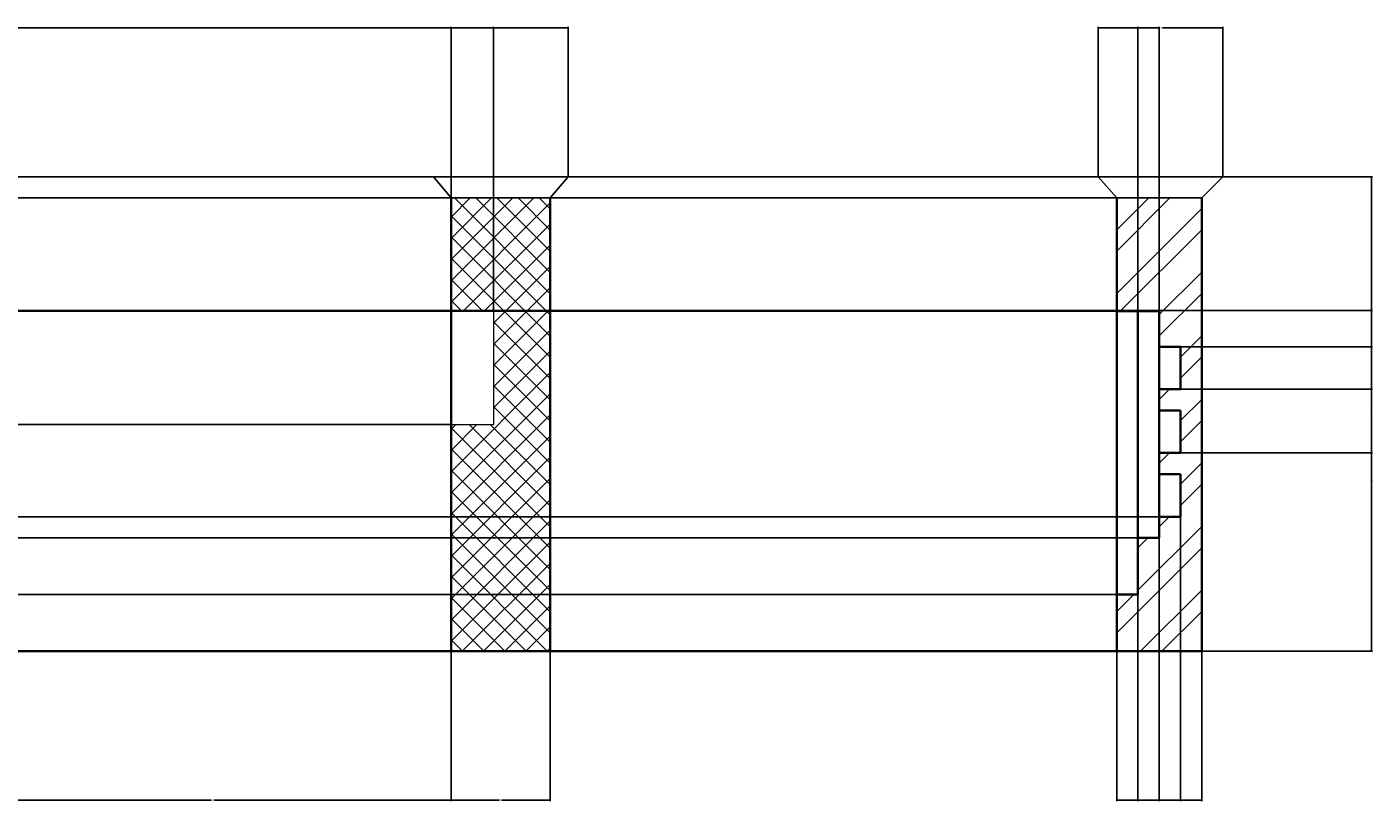
# Model space of a CAD drawing. Units: inches. Extents: x 2121 to 2815, y 1818 to 2233.
# Tile 5 of 6: x 2530 to 2815, y 1818 to 1982. Entities that reach past the tile are written whole.
import ezdxf

# ---------------------------------------------------------------- set-up
doc = ezdxf.new("R2010")
doc.units = ezdxf.units.IN
for name, color, linetype, lineweight in [('A-ANNO-DIMS', 2, 'Continuous', 18), ('A-COLS', 7, 'Continuous', 35), ('A-DETL', 7, 'Continuous', 18), ('A-ELEV-GRDE', 7, 'Continuous', 35), ('A-SECT', 7, 'Continuous', 35), ('A-WALL-COPG', 7, 'Continuous', 25), ('A-WALL-PATT', 8, 'Continuous', 13)]:
    doc.layers.add(name, color=color, linetype=linetype, lineweight=lineweight)
doc.styles.get("Standard").update_dxf_attribs({"font": 'arial.ttf'})
doc.dimstyles.get("Standard").update_dxf_attribs({"dimtxt": 0.18, "dimasz": 0.18, "dimexe": 0.18, "dimexo": 0.0625, "dimgap": 0.09, "dimtad": 0, "dimtih": 1, "dimtoh": 1, "dimdec": 4, "dimzin": 0, "dimdsep": 46, "dimtxsty": 'Standard', "dimcen": 0.09, "dimadec": 0, "dimazin": 0, "dimtfac": 1, "dimtdec": 4, "dimtofl": 0, "dimtmove": 0, "dimatfit": 3, "dimfxl": 1, "dimtolj": 1, "dimtzin": 0, "dimarcsym": 0})

# ---------------------------------------------------------------- blocks, each defined once
blk = doc.blocks.new('*D43')
at = {"layer": 'A-ANNO-DIMS', "color": 0, "lineweight": -2, "transparency": 16777216}
for p, q in [((2152.83, 1935.47), (2152.83, 1982.13)), ((2153.01, 1981.95), (2398.33, 1981.95)), ((2644.45, 1981.95), (2399.13, 1981.95)), ((2644.63, 1950.47), (2644.63, 1982.13))]:
    blk.add_line(p, q, dxfattribs=at)
at = {"layer": 'A-ANNO-DIMS', "color": 0, "transparency": 16777216}
for points in [[(2153.01, 1981.98), (2153.01, 1981.92), (2152.83, 1981.95)], [(2644.45, 1981.98), (2644.45, 1981.92), (2644.63, 1981.95)]]:
    blk.add_solid(points, dxfattribs=at)
at = {"layer": 'Defpoints', "color": 0, "transparency": 16777216}
for p in [(2644.63, 1981.95), (2644.63, 1950.41), (2152.83, 1935.41)]:
    blk.add_point(p, dxfattribs=at)
at = {"layer": 'A-ANNO-DIMS', "color": 0, "transparency": 16777216, "insert": (2398.73, 1981.95), "char_height": 0.18, "attachment_point": 5}
blk.add_mtext('\\A1;491.8', dxfattribs=at)
blk = doc.blocks.new('*D44')
at = {"layer": 'A-ANNO-DIMS', "color": 0, "lineweight": -2, "transparency": 16777216}
for p, q in [((2644.69, 1950.41), (2815, 1950.41)), ((2814.82, 1950.23), (2814.82, 1900.34)), ((2814.82, 1850.09), (2814.82, 1899.98)), ((2640.9, 1849.91), (2815, 1849.91))]:
    blk.add_line(p, q, dxfattribs=at)
at = {"layer": 'A-ANNO-DIMS', "color": 0, "transparency": 16777216}
for points in [[(2814.79, 1950.23), (2814.85, 1950.23), (2814.82, 1950.41)], [(2814.79, 1850.09), (2814.85, 1850.09), (2814.82, 1849.91)]]:
    blk.add_solid(points, dxfattribs=at)
at = {"layer": 'Defpoints', "color": 0, "transparency": 16777216}
for p in [(2644.63, 1950.41), (2814.82, 1950.41), (2640.83, 1849.91)]:
    blk.add_point(p, dxfattribs=at)
at = {"layer": 'A-ANNO-DIMS', "color": 0, "transparency": 16777216, "insert": (2814.82, 1900.16), "char_height": 0.18, "attachment_point": 5}
blk.add_mtext('\\A1;100.5', dxfattribs=at)
blk = doc.blocks.new('*D57')
at = {"layer": 'A-ANNO-DIMS', "color": 0, "lineweight": -2, "transparency": 16777216}
for p, q in [((2518.83, 1849.84), (2518.83, 1818.19)), ((2619.83, 1849.84), (2619.83, 1818.19)), ((2519.01, 1818.37), (2569.07, 1818.37)), ((2619.65, 1818.37), (2569.6, 1818.37))]:
    blk.add_line(p, q, dxfattribs=at)
at = {"layer": 'A-ANNO-DIMS', "color": 0, "transparency": 16777216}
for points in [[(2519.01, 1818.4), (2519.01, 1818.34), (2518.83, 1818.37)], [(2619.65, 1818.4), (2619.65, 1818.34), (2619.83, 1818.37)]]:
    blk.add_solid(points, dxfattribs=at)
at = {"layer": 'Defpoints', "color": 0, "transparency": 16777216}
for p in [(2518.83, 1849.91), (2619.83, 1849.91), (2619.83, 1818.37)]:
    blk.add_point(p, dxfattribs=at)
at = {"layer": 'A-ANNO-DIMS', "color": 0, "transparency": 16777216, "insert": (2569.33, 1818.37), "char_height": 0.18, "attachment_point": 5}
blk.add_mtext('\\A1;101', dxfattribs=at)
blk = doc.blocks.new('*D58')
at = {"layer": 'A-ANNO-DIMS', "color": 0, "lineweight": -2, "transparency": 16777216}
for p, q in [((2619.83, 1849.84), (2619.83, 1818.19)), ((2640.83, 1849.84), (2640.83, 1818.19)), ((2620.01, 1818.37), (2630.13, 1818.37)), ((2640.65, 1818.37), (2630.54, 1818.37))]:
    blk.add_line(p, q, dxfattribs=at)
at = {"layer": 'A-ANNO-DIMS', "color": 0, "transparency": 16777216}
for points in [[(2620.01, 1818.4), (2620.01, 1818.34), (2619.83, 1818.37)], [(2640.65, 1818.4), (2640.65, 1818.34), (2640.83, 1818.37)]]:
    blk.add_solid(points, dxfattribs=at)
at = {"layer": 'Defpoints', "color": 0, "transparency": 16777216}
for p in [(2619.83, 1849.91), (2640.83, 1849.91), (2640.83, 1818.37)]:
    blk.add_point(p, dxfattribs=at)
at = {"layer": 'A-ANNO-DIMS', "color": 0, "transparency": 16777216, "insert": (2630.33, 1818.37), "char_height": 0.18, "attachment_point": 5}
blk.add_mtext('\\A1;21', dxfattribs=at)
blk = doc.blocks.new('*D59')
at = {"layer": 'A-ANNO-DIMS', "color": 0, "lineweight": -2, "transparency": 16777216}
for p, q in [((2182.9, 1922.1), (2815, 1922.1)), ((2814.82, 1921.92), (2814.82, 1886.18)), ((2814.82, 1850.09), (2814.82, 1885.82)), ((2182.9, 1849.91), (2815, 1849.91))]:
    blk.add_line(p, q, dxfattribs=at)
at = {"layer": 'A-ANNO-DIMS', "color": 0, "transparency": 16777216}
for points in [[(2814.79, 1921.92), (2814.85, 1921.92), (2814.82, 1922.1)], [(2814.79, 1850.09), (2814.85, 1850.09), (2814.82, 1849.91)]]:
    blk.add_solid(points, dxfattribs=at)
at = {"layer": 'Defpoints', "color": 0, "transparency": 16777216}
for p in [(2182.83, 1922.1), (2814.82, 1922.1), (2182.83, 1849.91)]:
    blk.add_point(p, dxfattribs=at)
at = {"layer": 'A-ANNO-DIMS', "color": 0, "transparency": 16777216, "insert": (2814.82, 1886), "char_height": 0.18, "attachment_point": 5}
blk.add_mtext('\\A1;72.2', dxfattribs=at)
blk = doc.blocks.new('*D65')
at = {"layer": 'A-ANNO-DIMS', "color": 0, "lineweight": -2, "transparency": 16777216}
for p, q in [((2619.77, 1897.91), (2121.11, 1897.91)), ((2121.29, 1897.73), (2121.29, 1874.09)), ((2121.29, 1850.09), (2121.29, 1873.73)), ((2619.77, 1849.91), (2121.11, 1849.91))]:
    blk.add_line(p, q, dxfattribs=at)
at = {"layer": 'A-ANNO-DIMS', "color": 0, "transparency": 16777216}
for points in [[(2121.26, 1897.73), (2121.32, 1897.73), (2121.29, 1897.91)], [(2121.26, 1850.09), (2121.32, 1850.09), (2121.29, 1849.91)]]:
    blk.add_solid(points, dxfattribs=at)
at = {"layer": 'Defpoints', "color": 0, "transparency": 16777216}
for p in [(2121.29, 1897.91), (2619.83, 1897.91), (2619.83, 1849.91)]:
    blk.add_point(p, dxfattribs=at)
at = {"layer": 'A-ANNO-DIMS', "color": 0, "transparency": 16777216, "insert": (2121.29, 1873.91), "char_height": 0.18, "attachment_point": 5}
blk.add_mtext('\\A1;48', dxfattribs=at)
blk = doc.blocks.new('*D66')
at = {"layer": 'A-ANNO-DIMS', "color": 0, "lineweight": -2, "transparency": 16777216}
for p, q in [((2619.77, 1921.91), (2121.11, 1921.91)), ((2121.29, 1921.73), (2121.29, 1910.09)), ((2121.29, 1898.09), (2121.29, 1909.73)), ((2619.77, 1897.91), (2121.11, 1897.91))]:
    blk.add_line(p, q, dxfattribs=at)
at = {"layer": 'A-ANNO-DIMS', "color": 0, "transparency": 16777216}
for points in [[(2121.26, 1921.73), (2121.32, 1921.73), (2121.29, 1921.91)], [(2121.26, 1898.09), (2121.32, 1898.09), (2121.29, 1897.91)]]:
    blk.add_solid(points, dxfattribs=at)
at = {"layer": 'Defpoints', "color": 0, "transparency": 16777216}
for p in [(2121.29, 1921.91), (2619.83, 1921.91), (2619.83, 1897.91)]:
    blk.add_point(p, dxfattribs=at)
at = {"layer": 'A-ANNO-DIMS', "color": 0, "transparency": 16777216, "insert": (2121.29, 1909.91), "char_height": 0.18, "attachment_point": 5}
blk.add_mtext('\\A1;24', dxfattribs=at)
blk = doc.blocks.new('*D67')
at = {"layer": 'A-ANNO-DIMS', "color": 0, "lineweight": -2, "transparency": 16777216}
for p, q in [((2619.83, 1921.97), (2619.83, 1982.13)), ((2620.01, 1981.95), (2624.18, 1981.95)), ((2628.65, 1981.95), (2624.48, 1981.95)), ((2628.83, 1921.97), (2628.83, 1982.13))]:
    blk.add_line(p, q, dxfattribs=at)
at = {"layer": 'A-ANNO-DIMS', "color": 0, "transparency": 16777216}
for points in [[(2620.01, 1981.98), (2620.01, 1981.92), (2619.83, 1981.95)], [(2628.65, 1981.98), (2628.65, 1981.92), (2628.83, 1981.95)]]:
    blk.add_solid(points, dxfattribs=at)
at = {"layer": 'Defpoints', "color": 0, "transparency": 16777216}
for p in [(2628.83, 1981.95), (2619.83, 1921.91), (2628.83, 1921.91)]:
    blk.add_point(p, dxfattribs=at)
at = {"layer": 'A-ANNO-DIMS', "color": 0, "transparency": 16777216, "insert": (2624.33, 1981.95), "char_height": 0.18, "attachment_point": 5}
blk.add_mtext('\\A1;9', dxfattribs=at)
blk = doc.blocks.new('*D69')
at = {"layer": 'A-ANNO-DIMS', "color": 0, "lineweight": -2, "transparency": 16777216}
for p, q in [((2760.83, 1849.84), (2760.83, 1818.19)), ((2778.83, 1849.84), (2778.83, 1818.19)), ((2761.01, 1818.37), (2769.62, 1818.37)), ((2778.65, 1818.37), (2770.04, 1818.37))]:
    blk.add_line(p, q, dxfattribs=at)
at = {"layer": 'A-ANNO-DIMS', "color": 0, "transparency": 16777216}
for points in [[(2761.01, 1818.4), (2761.01, 1818.34), (2760.83, 1818.37)], [(2778.65, 1818.4), (2778.65, 1818.34), (2778.83, 1818.37)]]:
    blk.add_solid(points, dxfattribs=at)
at = {"layer": 'Defpoints', "color": 0, "transparency": 16777216}
for p in [(2760.83, 1849.91), (2778.83, 1849.91), (2778.83, 1818.37)]:
    blk.add_point(p, dxfattribs=at)
at = {"layer": 'A-ANNO-DIMS', "color": 0, "transparency": 16777216, "insert": (2769.83, 1818.37), "char_height": 0.18, "attachment_point": 5}
blk.add_mtext('\\A1;18', dxfattribs=at)
blk = doc.blocks.new('*D70')
at = {"layer": 'A-ANNO-DIMS', "color": 0, "lineweight": -2, "transparency": 16777216}
for p, q in [((2756.93, 1950.47), (2756.93, 1982.13)), ((2757.11, 1981.95), (2769.71, 1981.95)), ((2783.1, 1981.95), (2770.5, 1981.95)), ((2783.28, 1950.47), (2783.28, 1982.13))]:
    blk.add_line(p, q, dxfattribs=at)
at = {"layer": 'A-ANNO-DIMS', "color": 0, "transparency": 16777216}
for points in [[(2757.11, 1981.98), (2757.11, 1981.92), (2756.93, 1981.95)], [(2783.1, 1981.98), (2783.1, 1981.92), (2783.28, 1981.95)]]:
    blk.add_solid(points, dxfattribs=at)
at = {"layer": 'Defpoints', "color": 0, "transparency": 16777216}
for p in [(2783.28, 1981.95), (2756.93, 1950.41), (2783.28, 1950.41)]:
    blk.add_point(p, dxfattribs=at)
at = {"layer": 'A-ANNO-DIMS', "color": 0, "transparency": 16777216, "insert": (2770.11, 1981.95), "char_height": 0.18, "attachment_point": 5}
blk.add_mtext('\\A1;26.35', dxfattribs=at)
blk = doc.blocks.new('*D71')
at = {"layer": 'A-ANNO-DIMS', "color": 0, "lineweight": -2, "transparency": 16777216}
for p, q in [((2783.34, 1950.41), (2815, 1950.41)), ((2814.82, 1950.23), (2814.82, 1900.34)), ((2814.82, 1850.09), (2814.82, 1899.98)), ((2778.9, 1849.91), (2815, 1849.91))]:
    blk.add_line(p, q, dxfattribs=at)
at = {"layer": 'A-ANNO-DIMS', "color": 0, "transparency": 16777216}
for points in [[(2814.79, 1950.23), (2814.85, 1950.23), (2814.82, 1950.41)], [(2814.79, 1850.09), (2814.85, 1850.09), (2814.82, 1849.91)]]:
    blk.add_solid(points, dxfattribs=at)
at = {"layer": 'Defpoints', "color": 0, "transparency": 16777216}
for p in [(2783.28, 1950.41), (2814.82, 1950.41), (2778.83, 1849.91)]:
    blk.add_point(p, dxfattribs=at)
at = {"layer": 'A-ANNO-DIMS', "color": 0, "transparency": 16777216, "insert": (2814.82, 1900.16), "char_height": 0.18, "attachment_point": 5}
blk.add_mtext('\\A1;100.5', dxfattribs=at)
blk = doc.blocks.new('*D72')
at = {"layer": 'A-ANNO-DIMS', "color": 0, "lineweight": -2, "transparency": 16777216}
for p, q in [((2760.77, 1861.91), (2121.11, 1861.91)), ((2121.29, 1861.73), (2121.29, 1856.09)), ((2121.29, 1850.09), (2121.29, 1855.73)), ((2760.77, 1849.91), (2121.11, 1849.91))]:
    blk.add_line(p, q, dxfattribs=at)
at = {"layer": 'A-ANNO-DIMS', "color": 0, "transparency": 16777216}
for points in [[(2121.26, 1861.73), (2121.32, 1861.73), (2121.29, 1861.91)], [(2121.26, 1850.09), (2121.32, 1850.09), (2121.29, 1849.91)]]:
    blk.add_solid(points, dxfattribs=at)
at = {"layer": 'Defpoints', "color": 0, "transparency": 16777216}
for p in [(2121.29, 1861.91), (2760.83, 1861.91), (2760.83, 1849.91)]:
    blk.add_point(p, dxfattribs=at)
at = {"layer": 'A-ANNO-DIMS', "color": 0, "transparency": 16777216, "insert": (2121.29, 1855.91), "char_height": 0.18, "attachment_point": 5}
blk.add_mtext('\\A1;12', dxfattribs=at)
blk = doc.blocks.new('*D73')
at = {"layer": 'A-ANNO-DIMS', "color": 0, "lineweight": -2, "transparency": 16777216}
for p, q in [((2765.27, 1873.91), (2121.11, 1873.91)), ((2121.29, 1873.73), (2121.29, 1868.09)), ((2121.29, 1862.09), (2121.29, 1867.73)), ((2760.77, 1861.91), (2121.11, 1861.91))]:
    blk.add_line(p, q, dxfattribs=at)
at = {"layer": 'A-ANNO-DIMS', "color": 0, "transparency": 16777216}
for points in [[(2121.26, 1873.73), (2121.32, 1873.73), (2121.29, 1873.91)], [(2121.26, 1862.09), (2121.32, 1862.09), (2121.29, 1861.91)]]:
    blk.add_solid(points, dxfattribs=at)
at = {"layer": 'Defpoints', "color": 0, "transparency": 16777216}
for p in [(2121.29, 1873.91), (2765.33, 1873.91), (2760.83, 1861.91)]:
    blk.add_point(p, dxfattribs=at)
at = {"layer": 'A-ANNO-DIMS', "color": 0, "transparency": 16777216, "insert": (2121.29, 1867.91), "char_height": 0.18, "attachment_point": 5}
blk.add_mtext('\\A1;12', dxfattribs=at)
blk = doc.blocks.new('*D74')
at = {"layer": 'A-ANNO-DIMS', "color": 0, "lineweight": -2, "transparency": 16777216}
for p, q in [((2765.27, 1921.91), (2121.11, 1921.91)), ((2121.29, 1921.73), (2121.29, 1898.09)), ((2121.29, 1874.09), (2121.29, 1897.73)), ((2765.27, 1873.91), (2121.11, 1873.91))]:
    blk.add_line(p, q, dxfattribs=at)
at = {"layer": 'A-ANNO-DIMS', "color": 0, "transparency": 16777216}
for points in [[(2121.26, 1921.73), (2121.32, 1921.73), (2121.29, 1921.91)], [(2121.26, 1874.09), (2121.32, 1874.09), (2121.29, 1873.91)]]:
    blk.add_solid(points, dxfattribs=at)
at = {"layer": 'Defpoints', "color": 0, "transparency": 16777216}
for p in [(2121.29, 1921.91), (2765.33, 1921.91), (2765.33, 1873.91)]:
    blk.add_point(p, dxfattribs=at)
at = {"layer": 'A-ANNO-DIMS', "color": 0, "transparency": 16777216, "insert": (2121.29, 1897.91), "char_height": 0.18, "attachment_point": 5}
blk.add_mtext('\\A1;48', dxfattribs=at)
blk = doc.blocks.new('*D75')
at = {"layer": 'A-ANNO-DIMS', "color": 0, "lineweight": -2, "transparency": 16777216}
for p, q in [((2760.77, 1945.91), (2121.11, 1945.91)), ((2121.29, 1945.73), (2121.29, 1934.09)), ((2121.29, 1922.09), (2121.29, 1933.73)), ((2760.77, 1921.91), (2121.11, 1921.91))]:
    blk.add_line(p, q, dxfattribs=at)
at = {"layer": 'A-ANNO-DIMS', "color": 0, "transparency": 16777216}
for points in [[(2121.26, 1945.73), (2121.32, 1945.73), (2121.29, 1945.91)], [(2121.26, 1922.09), (2121.32, 1922.09), (2121.29, 1921.91)]]:
    blk.add_solid(points, dxfattribs=at)
at = {"layer": 'Defpoints', "color": 0, "transparency": 16777216}
for p in [(2121.29, 1945.91), (2760.83, 1945.91), (2760.83, 1921.91)]:
    blk.add_point(p, dxfattribs=at)
at = {"layer": 'A-ANNO-DIMS', "color": 0, "transparency": 16777216, "insert": (2121.29, 1933.91), "char_height": 0.18, "attachment_point": 5}
blk.add_mtext('\\A1;24', dxfattribs=at)
blk = doc.blocks.new('*D76')
at = {"layer": 'A-ANNO-DIMS', "color": 0, "lineweight": -2, "transparency": 16777216}
for p, q in [((2756.87, 1950.41), (2121.11, 1950.41)), ((2121.29, 1950.23), (2121.29, 1948.34)), ((2121.29, 1946.09), (2121.29, 1947.98)), ((2760.77, 1945.91), (2121.11, 1945.91))]:
    blk.add_line(p, q, dxfattribs=at)
at = {"layer": 'A-ANNO-DIMS', "color": 0, "transparency": 16777216}
for points in [[(2121.26, 1950.23), (2121.32, 1950.23), (2121.29, 1950.41)], [(2121.26, 1946.09), (2121.32, 1946.09), (2121.29, 1945.91)]]:
    blk.add_solid(points, dxfattribs=at)
at = {"layer": 'Defpoints', "color": 0, "transparency": 16777216}
for p in [(2121.29, 1950.41), (2756.93, 1950.41), (2760.83, 1945.91)]:
    blk.add_point(p, dxfattribs=at)
at = {"layer": 'A-ANNO-DIMS', "color": 0, "transparency": 16777216, "insert": (2121.29, 1948.16), "char_height": 0.18, "attachment_point": 5}
blk.add_mtext('\\A1;4.5', dxfattribs=at)
blk = doc.blocks.new('*D77')
at = {"layer": 'A-ANNO-DIMS', "color": 0, "lineweight": -2, "transparency": 16777216}
for p, q in [((2760.83, 1861.84), (2760.83, 1818.19)), ((2765.33, 1861.84), (2765.33, 1818.19)), ((2761.01, 1818.37), (2762.82, 1818.37)), ((2765.15, 1818.37), (2763.34, 1818.37))]:
    blk.add_line(p, q, dxfattribs=at)
at = {"layer": 'A-ANNO-DIMS', "color": 0, "transparency": 16777216}
for points in [[(2761.01, 1818.4), (2761.01, 1818.34), (2760.83, 1818.37)], [(2765.15, 1818.4), (2765.15, 1818.34), (2765.33, 1818.37)]]:
    blk.add_solid(points, dxfattribs=at)
at = {"layer": 'Defpoints', "color": 0, "transparency": 16777216}
for p in [(2760.83, 1861.91), (2765.33, 1861.91), (2765.33, 1818.37)]:
    blk.add_point(p, dxfattribs=at)
at = {"layer": 'A-ANNO-DIMS', "color": 0, "transparency": 16777216, "insert": (2763.08, 1818.37), "char_height": 0.18, "attachment_point": 5}
blk.add_mtext('\\A1;4.5', dxfattribs=at)
blk = doc.blocks.new('*D78')
at = {"layer": 'A-ANNO-DIMS', "color": 0, "lineweight": -2, "transparency": 16777216}
for p, q in [((2765.33, 1921.97), (2765.33, 1982.13)), ((2765.51, 1981.95), (2767.32, 1981.95)), ((2769.65, 1981.95), (2767.84, 1981.95)), ((2769.83, 1921.97), (2769.83, 1982.13))]:
    blk.add_line(p, q, dxfattribs=at)
at = {"layer": 'A-ANNO-DIMS', "color": 0, "transparency": 16777216}
for points in [[(2765.51, 1981.98), (2765.51, 1981.92), (2765.33, 1981.95)], [(2769.65, 1981.98), (2769.65, 1981.92), (2769.83, 1981.95)]]:
    blk.add_solid(points, dxfattribs=at)
at = {"layer": 'Defpoints', "color": 0, "transparency": 16777216}
for p in [(2769.83, 1981.95), (2765.33, 1921.91), (2769.83, 1921.91)]:
    blk.add_point(p, dxfattribs=at)
at = {"layer": 'A-ANNO-DIMS', "color": 0, "transparency": 16777216, "insert": (2767.58, 1981.95), "char_height": 0.18, "attachment_point": 5}
blk.add_mtext('\\A1;4.5', dxfattribs=at)
blk = doc.blocks.new('*D79')
at = {"layer": 'A-ANNO-DIMS', "color": 0, "lineweight": -2, "transparency": 16777216}
for p, q in [((2769.83, 1878.34), (2769.83, 1818.19)), ((2774.33, 1878.34), (2774.33, 1818.19)), ((2770.01, 1818.37), (2771.82, 1818.37)), ((2774.15, 1818.37), (2772.34, 1818.37))]:
    blk.add_line(p, q, dxfattribs=at)
at = {"layer": 'A-ANNO-DIMS', "color": 0, "transparency": 16777216}
for points in [[(2770.01, 1818.4), (2770.01, 1818.34), (2769.83, 1818.37)], [(2774.15, 1818.4), (2774.15, 1818.34), (2774.33, 1818.37)]]:
    blk.add_solid(points, dxfattribs=at)
at = {"layer": 'Defpoints', "color": 0, "transparency": 16777216}
for p in [(2769.83, 1878.41), (2774.33, 1878.41), (2774.33, 1818.37)]:
    blk.add_point(p, dxfattribs=at)
at = {"layer": 'A-ANNO-DIMS', "color": 0, "transparency": 16777216, "insert": (2772.08, 1818.37), "char_height": 0.18, "attachment_point": 5}
blk.add_mtext('\\A1;4.5', dxfattribs=at)
blk = doc.blocks.new('*D80')
at = {"layer": 'A-ANNO-DIMS', "color": 0, "lineweight": -2, "transparency": 16777216}
for p, q in [((2774.4, 1914.41), (2815, 1914.41)), ((2814.82, 1914.23), (2814.82, 1910.09)), ((2814.82, 1905.59), (2814.82, 1909.73)), ((2774.4, 1905.41), (2815, 1905.41))]:
    blk.add_line(p, q, dxfattribs=at)
at = {"layer": 'A-ANNO-DIMS', "color": 0, "transparency": 16777216}
for points in [[(2814.79, 1914.23), (2814.85, 1914.23), (2814.82, 1914.41)], [(2814.79, 1905.59), (2814.85, 1905.59), (2814.82, 1905.41)]]:
    blk.add_solid(points, dxfattribs=at)
at = {"layer": 'Defpoints', "color": 0, "transparency": 16777216}
for p in [(2774.33, 1914.41), (2814.82, 1914.41), (2774.33, 1905.41)]:
    blk.add_point(p, dxfattribs=at)
at = {"layer": 'A-ANNO-DIMS', "color": 0, "transparency": 16777216, "insert": (2814.82, 1909.91), "char_height": 0.18, "attachment_point": 5}
blk.add_mtext('\\A1;9', dxfattribs=at)
blk = doc.blocks.new('*D81')
at = {"layer": 'A-ANNO-DIMS', "color": 0, "lineweight": -2, "transparency": 16777216}
for p, q in [((2774.4, 1905.41), (2815, 1905.41)), ((2814.82, 1905.23), (2814.82, 1898.84)), ((2814.82, 1892.09), (2814.82, 1898.48)), ((2774.4, 1891.91), (2815, 1891.91))]:
    blk.add_line(p, q, dxfattribs=at)
at = {"layer": 'A-ANNO-DIMS', "color": 0, "transparency": 16777216}
for points in [[(2814.79, 1905.23), (2814.85, 1905.23), (2814.82, 1905.41)], [(2814.79, 1892.09), (2814.85, 1892.09), (2814.82, 1891.91)]]:
    blk.add_solid(points, dxfattribs=at)
at = {"layer": 'Defpoints', "color": 0, "transparency": 16777216}
for p in [(2774.33, 1905.41), (2814.82, 1905.41), (2774.33, 1891.91)]:
    blk.add_point(p, dxfattribs=at)
at = {"layer": 'A-ANNO-DIMS', "color": 0, "transparency": 16777216, "insert": (2814.82, 1898.66), "char_height": 0.18, "attachment_point": 5}
blk.add_mtext('\\A1;13.5', dxfattribs=at)
blk = doc.blocks.new('*D82')
at = {"layer": 'A-ANNO-DIMS', "color": 0, "lineweight": -2, "transparency": 16777216}
for p, q in [((2769.77, 1878.41), (2121.11, 1878.41)), ((2121.29, 1878.23), (2121.29, 1876.34)), ((2769.77, 1873.91), (2121.11, 1873.91)), ((2121.29, 1874.09), (2121.29, 1875.98))]:
    blk.add_line(p, q, dxfattribs=at)
at = {"layer": 'A-ANNO-DIMS', "color": 0, "transparency": 16777216}
for points in [[(2121.26, 1878.23), (2121.32, 1878.23), (2121.29, 1878.41)], [(2121.26, 1874.09), (2121.32, 1874.09), (2121.29, 1873.91)]]:
    blk.add_solid(points, dxfattribs=at)
at = {"layer": 'Defpoints', "color": 0, "transparency": 16777216}
for p in [(2121.29, 1878.41), (2769.83, 1878.41), (2769.83, 1873.91)]:
    blk.add_point(p, dxfattribs=at)
at = {"layer": 'A-ANNO-DIMS', "color": 0, "transparency": 16777216, "insert": (2121.29, 1876.16), "char_height": 0.18, "attachment_point": 5}
blk.add_mtext('\\A1;4.5', dxfattribs=at)

msp = doc.modelspace()

# ---------------------------------------------------------------- hatches: boundary and pattern name
at = {"layer": 'A-WALL-PATT'}
h = msp.add_hatch(dxfattribs=at)
h.set_pattern_fill('ANSI37', color=256)
h.paths.add_polyline_path([(2518.8326, 1945.9075), (2494.8326, 1945.9075), (2494.8326, 1849.9075), (2503.8326, 1849.9075), (2518.8326, 1849.9075), (2518.8326, 1897.9075), (2503.8326, 1897.9075), (2503.8326, 1921.9075), (2518.8326, 1921.9075)])
h.paths.add_polyline_path([(2640.8326, 1945.9075), (2619.8326, 1945.9075), (2619.8326, 1921.9075), (2628.8326, 1921.9075), (2628.8326, 1897.9075), (2619.8326, 1897.9075), (2619.8326, 1849.9075), (2640.8326, 1849.9075)])
h = msp.add_hatch(dxfattribs=at)
h.set_pattern_fill('ANSI32', color=256)
h.paths.add_polyline_path([(2778.8326, 1945.9075), (2760.8326, 1945.9075), (2760.8326, 1921.9075), (2769.8326, 1921.9075), (2769.8326, 1914.4075), (2774.3326, 1914.4075), (2774.3326, 1905.4075), (2769.8326, 1905.4075), (2769.8326, 1900.9075), (2774.3326, 1900.9075), (2774.3326, 1891.9075), (2769.8326, 1891.9075), (2769.8326, 1887.4075), (2774.3326, 1887.4075), (2774.3326, 1878.4075), (2769.8326, 1878.4075), (2769.8326, 1873.9075), (2765.3326, 1873.9075), (2765.3326, 1861.9075), (2760.8326, 1861.9075), (2760.8326, 1849.9075), (2778.8326, 1849.9075)])

# ---------------------------------------------------------------- linework, layer by layer
at = {"layer": 'A-COLS'}
for p, q in [((2619.8326, 1849.9075), (2619.8326, 1945.9075)), ((2640.8326, 1849.9075), (2640.8326, 1945.9075)), ((2640.8326, 1870.9178), (2640.8326, 1849.9075))]:
    msp.add_line(p, q, dxfattribs=at)
at = {"layer": 'A-DETL'}
for p, q in [((2619.8326, 1921.9075), (2628.8326, 1921.9075)), ((2628.8326, 1921.9075), (2628.8326, 1897.9075)), ((2619.8326, 1897.9075), (2628.8326, 1897.9075))]:
    msp.add_line(p, q, dxfattribs=at)
at = {"layer": 'A-ELEV-GRDE'}
for p, q in [((2152.8326, 1849.9075), (2778.8326, 1849.9075)), ((2518.8326, 1849.9075), (2619.8326, 1849.9075)), ((2640.8326, 1849.9075), (2760.8326, 1849.9075))]:
    msp.add_line(p, q, dxfattribs=at)
at = {"layer": 'A-SECT'}
for p, q in [((2760.8326, 1849.9075), (2760.8326, 1945.9075)), ((2778.8326, 1849.9075), (2778.8326, 1945.9075)), ((2760.8326, 1921.9075), (2769.8326, 1921.9075)), ((2765.3326, 1861.9075), (2765.3326, 1921.9075)), ((2769.8326, 1921.9075), (2769.8326, 1873.9075)), ((2774.3326, 1914.4075), (2769.8326, 1914.4075)), ((2774.3326, 1905.4075), (2774.3326, 1914.4075)), ((2769.8326, 1900.9075), (2769.8326, 1905.4075)), ((2769.8326, 1905.4075), (2774.3326, 1905.4075)), ((2774.3326, 1900.9075), (2769.8326, 1900.9075)), ((2774.3326, 1891.9075), (2774.3326, 1900.9075)), ((2769.8326, 1887.4075), (2769.8326, 1891.9075)), ((2769.8326, 1891.9075), (2774.3326, 1891.9075)), ((2774.3326, 1887.4075), (2769.8326, 1887.4075)), ((2774.3326, 1878.4075), (2774.3326, 1887.4075)), ((2769.8326, 1873.9075), (2769.8326, 1878.4075)), ((2769.8326, 1878.4075), (2774.3326, 1878.4075)), ((2778.8326, 1878.4075), (2778.8326, 1849.9075)), ((2769.8326, 1873.9075), (2765.3326, 1873.9075)), ((2760.8326, 1849.9075), (2760.8326, 1861.9075)), ((2760.8326, 1861.9075), (2765.3326, 1861.9075))]:
    msp.add_line(p, q, dxfattribs=at)
at = {"layer": 'A-WALL-COPG'}
for p, q in [((2619.8326, 1945.9075), (2616.1211, 1950.4075)), ((2616.1211, 1950.4075), (2644.6318, 1950.4075)), ((2640.8326, 1945.9075), (2644.6318, 1950.4075)), ((2760.8326, 1945.9075), (2756.9306, 1950.4075)), ((2756.9306, 1950.4075), (2783.28, 1950.4075)), ((2778.8326, 1945.9075), (2783.28, 1950.4075)), ((2619.8326, 1945.9075), (2640.8326, 1945.9075)), ((2760.8326, 1945.9075), (2778.8326, 1945.9075))]:
    msp.add_line(p, q, dxfattribs=at)

# ---------------------------------------------------------------- dimensions: what is measured, and where the dimension line sits
at = {"layer": 'A-ANNO-DIMS'}
for base, p1, p2, override, picture, middle in [((2644.6318, 1981.9475), (2152.8326, 1935.4075), (2644.6318, 1950.4075), {"dimdec": 1, "dimlfac": 1, "dimrnd": 0, "dimzin": 0, "dimdsep": 46, "dimlunit": 2}, '*D43', (2398.7322, 1981.9475)), ((2628.8326, 1981.9475), (2619.8326, 1921.9075), (2628.8326, 1921.9075), {"dimdec": 0, "dimlfac": 1, "dimrnd": 0, "dimzin": 0, "dimdsep": 46, "dimlunit": 2}, '*D67', (2624.3326, 1981.9475)), ((2783.28, 1981.9475), (2756.9306, 1950.4075), (2783.28, 1950.4075), {"dimdec": 2, "dimlfac": 1, "dimrnd": 0, "dimzin": 0, "dimdsep": 46, "dimlunit": 2}, '*D70', (2770.1053, 1981.9475)), ((2769.8326, 1981.9475), (2765.3326, 1921.9075), (2769.8326, 1921.9075), {"dimdec": 1, "dimlfac": 1, "dimrnd": 0, "dimzin": 0, "dimdsep": 46, "dimlunit": 2}, '*D78', (2767.5826, 1981.9475)), ((2774.3326, 1818.3675), (2769.8326, 1878.4075), (2774.3326, 1878.4075), {"dimdec": 1, "dimlfac": 1, "dimrnd": 0, "dimzin": 0, "dimdsep": 46, "dimlunit": 2}, '*D79', (2772.0826, 1818.3675)), ((2765.3326, 1818.3675), (2760.8326, 1861.9075), (2765.3326, 1861.9075), {"dimdec": 1, "dimlfac": 1, "dimrnd": 0, "dimzin": 0, "dimdsep": 46, "dimlunit": 2}, '*D77', (2763.0826, 1818.3675)), ((2619.8326, 1818.3675), (2518.8326, 1849.9075), (2619.8326, 1849.9075), {"dimdec": 0, "dimlfac": 1, "dimrnd": 0, "dimzin": 0, "dimdsep": 46, "dimlunit": 2}, '*D57', (2569.3326, 1818.3675)), ((2640.8326, 1818.3675), (2619.8326, 1849.9075), (2640.8326, 1849.9075), {"dimdec": 0, "dimlfac": 1, "dimrnd": 0, "dimzin": 0, "dimdsep": 46, "dimlunit": 2}, '*D58', (2630.3326, 1818.3675)), ((2778.8326, 1818.3675), (2760.8326, 1849.9075), (2778.8326, 1849.9075), {"dimdec": 0, "dimlfac": 1, "dimrnd": 0, "dimzin": 0, "dimdsep": 46, "dimlunit": 2}, '*D69', (2769.8326, 1818.3675))]:
    dim = msp.add_linear_dim(base=base, p1=p1, p2=p2, dimstyle='Standard', override=override, dxfattribs=at)
    dim.commit()
    dim.dimension.update_dxf_attribs({"geometry": picture, "text_midpoint": middle})
for base, p1, p2, override, picture, middle in [((2121.2926, 1950.4075), (2760.8326, 1945.9075), (2756.9306, 1950.4075), {"dimdec": 1, "dimlfac": 1, "dimrnd": 0, "dimzin": 0, "dimdsep": 46, "dimlunit": 2}, '*D76', (2121.2926, 1948.1575)), ((2814.82, 1950.4075), (2640.8326, 1849.9075), (2644.6318, 1950.4075), {"dimdec": 1, "dimlfac": 1, "dimrnd": 0, "dimzin": 0, "dimdsep": 46, "dimlunit": 2}, '*D44', (2814.82, 1900.1575)), ((2814.82, 1950.4075), (2778.8326, 1849.9075), (2783.28, 1950.4075), {"dimdec": 1, "dimlfac": 1, "dimrnd": 0, "dimzin": 0, "dimdsep": 46, "dimlunit": 2}, '*D71', (2814.82, 1900.1575)), ((2121.2926, 1945.9075), (2760.8326, 1921.9075), (2760.8326, 1945.9075), {"dimdec": 0, "dimlfac": 1, "dimrnd": 0, "dimzin": 0, "dimdsep": 46, "dimlunit": 2}, '*D75', (2121.2926, 1933.9075)), ((2121.2926, 1921.9075), (2619.8326, 1897.9075), (2619.8326, 1921.9075), {"dimdec": 0, "dimlfac": 1, "dimrnd": 0, "dimzin": 0, "dimdsep": 46, "dimlunit": 2}, '*D66', (2121.2926, 1909.9075)), ((2121.2926, 1921.9075), (2765.3326, 1873.9075), (2765.3326, 1921.9075), {"dimdec": 0, "dimlfac": 1, "dimrnd": 0, "dimzin": 0, "dimdsep": 46, "dimlunit": 2}, '*D74', (2121.2926, 1897.9075)), ((2814.82, 1922.1005), (2182.8326, 1849.9075), (2182.8326, 1922.1005), {"dimdec": 1, "dimlfac": 1, "dimrnd": 0, "dimzin": 0, "dimdsep": 46, "dimlunit": 2}, '*D59', (2814.82, 1886.004)), ((2814.82, 1914.4075), (2774.3326, 1905.4075), (2774.3326, 1914.4075), {"dimdec": 0, "dimlfac": 1, "dimrnd": 0, "dimzin": 0, "dimdsep": 46, "dimlunit": 2}, '*D80', (2814.82, 1909.9075)), ((2814.82, 1905.4075), (2774.3326, 1891.9075), (2774.3326, 1905.4075), {"dimdec": 1, "dimlfac": 1, "dimrnd": 0, "dimzin": 0, "dimdsep": 46, "dimlunit": 2}, '*D81', (2814.82, 1898.6575)), ((2121.2926, 1897.9075), (2619.8326, 1849.9075), (2619.8326, 1897.9075), {"dimdec": 0, "dimlfac": 1, "dimrnd": 0, "dimzin": 0, "dimdsep": 46, "dimlunit": 2}, '*D65', (2121.2926, 1873.9075)), ((2121.2926, 1878.4075), (2769.8326, 1873.9075), (2769.8326, 1878.4075), {"dimdec": 1, "dimlfac": 1, "dimrnd": 0, "dimzin": 0, "dimdsep": 46, "dimlunit": 2}, '*D82', (2121.2926, 1876.1575)), ((2121.2926, 1873.9075), (2760.8326, 1861.9075), (2765.3326, 1873.9075), {"dimdec": 0, "dimlfac": 1, "dimrnd": 0, "dimzin": 0, "dimdsep": 46, "dimlunit": 2}, '*D73', (2121.2926, 1867.9075)), ((2121.2926, 1861.9075), (2760.8326, 1849.9075), (2760.8326, 1861.9075), {"dimdec": 0, "dimlfac": 1, "dimrnd": 0, "dimzin": 0, "dimdsep": 46, "dimlunit": 2}, '*D72', (2121.2926, 1855.9075))]:
    dim = msp.add_linear_dim(base=base, p1=p1, p2=p2, angle=90, dimstyle='Standard', override=override, dxfattribs=at)
    dim.commit()
    dim.dimension.update_dxf_attribs({"geometry": picture, "text_midpoint": middle})

doc.saveas('drawing.dxf')
